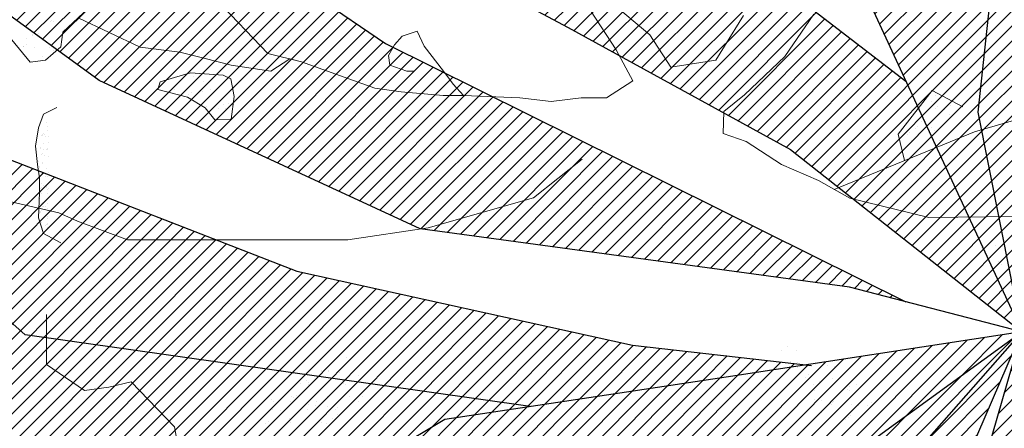
# Model space of a CAD drawing. Units: inches. Extents: x 1986 to 21484, y -1816 to 2016.
# Tile 20 of 85: x 2157.68 to 2172.01, y 1882.44 to 1888.38. Entities that reach past the tile are written whole.
import ezdxf

# ---------------------------------------------------------------- set-up
doc = ezdxf.new("R2010")
doc.units = ezdxf.units.IN
doc.layers.add('L-PLNT', color=84, linetype='Continuous', lineweight=13)
doc.layers.add('vfolhas', color=114, linetype='Continuous', lineweight=5)
for name, color, linetype in [('vfolha', 72, 'Continuous'), ('vfolha2', 110, 'Continuous'), ('vfolhas2', 102, 'Continuous')]:
    doc.layers.add(name, color=color, linetype=linetype)
pattern_1 = [(45, (-2446.5133113, 50.986076), (-0.004419417382, 0.004419417382), [])]

# ---------------------------------------------------------------- blocks, each defined once
blk = doc.blocks.new('arbusto_PB_verde_grande')
at = {"layer": 'vfolha2'}
h = blk.add_hatch(dxfattribs=at)
h.set_pattern_fill('ANSI31', color=256, scale=0.05, style=0)
h.set_pattern_definition(pattern_1)
h.paths.add_polyline_path([(0.02944, 0.35651), (0.00028, 0.09048), (0.02625, -0.03934), (0.047, 0.06233), (0.06189, 0.09731), (0.09372, 0.26573), (0.09955, 0.43473), (0.08789, 0.61313), (0.0645, 0.72266), (0.04988, 0.6851), (0.0236, 0.51294)])
h.paths.add_polyline_path([(0.30106, 0.43789), (0.14225, 0.24871), (0.26685, 0.30022)])
h.paths.add_polyline_path([(0.37995, 0.22817), (0.23697, 0.15193), (0.18428, 0.09364), (0.11122, 0.04358), (0.02625, -0.03934), (0.28061, 0.04667), (0.36829, 0.07798), (0.46756, 0.11239), (0.61068, 0.19376), (0.71585, 0.27823), (0.55813, 0.25948)])
h.paths.add_polyline_path([(0.56101, -0.29441), (0.72752, -0.32573), (0.59024, -0.2412), (0.42962, -0.15982), (0.02625, -0.03934), (0.14922, -0.14107), (0.18838, -0.16604), (0.41501, -0.24435)])
h.paths.add_polyline_path([(-0.27429, -0.44776), (-0.30352, -0.72628), (-0.23923, -0.64175), (-0.15457, -0.45716), (0.02625, -0.03934), (-0.16328, -0.25376)])
h.paths.add_polyline_path([(-0.51963, -0.24744), (-0.67736, -0.32573), (-0.59558, -0.35072), (-0.40574, -0.32882), (-0.21007, -0.20995), (0.02625, -0.03934), (-0.14874, -0.06595), (-0.31518, -0.09101), (-0.41452, -0.15048)])
h.paths.add_polyline_path([(-0.52546, 0.25007), (-0.70947, 0.24698), (-0.51963, 0.1093), (-0.32979, 0.02167), (-0.07567, -0.0128), (-0.04234, -0.02148), (-0.35024, 0.1312)])
at = {"layer": 'vfolhas'}
h = blk.add_hatch(dxfattribs=at)
h.set_pattern_fill('ANSI31', color=256, scale=0.05, style=0)
h.set_pattern_definition(pattern_1)
h.paths.add_polyline_path([(-0.07279, 0.50669), (-0.18085, 0.65063), (-0.2334, 0.67253), (-0.20712, 0.53176), (-0.10785, 0.25007), (0.02625, -0.03934), (0.00028, 0.09048), (0.00816, 0.16241), (-0.04939, 0.29079)])
h.paths.add_polyline_path([(0.09902, 0.41929), (0.09372, 0.26573), (0.07906, 0.18814), (0.15506, 0.36901), (0.26606, 0.5505), (0.28356, 0.63504), (0.2485, 0.68819), (0.25145, 0.63504), (0.20178, 0.54426)])
h.paths.add_polyline_path([(0.12295, 0.24073), (0.047, 0.06233), (0.02625, -0.03934), (0.11122, 0.04358), (0.18428, 0.09364), (0.27478, 0.19376), (0.3215, 0.25323), (0.44129, 0.38467), (0.47634, 0.57866), (0.41789, 0.45347), (0.28939, 0.30954)])
h.paths.add_polyline_path([(0.58145, -0.03779), (0.70707, 0.01536), (0.78591, 0.04667), (0.74796, 0.06549), (0.62818, 0.08423), (0.52595, 0.09048), (0.39745, 0.04358), (0.02625, -0.03934), (0.25728, -0.03154), (0.43834, -0.0347)])
h.paths.add_polyline_path([(0.52022, -0.03647), (0.43834, -0.0347), (0.25728, -0.03154), (0.02625, -0.03934), (0.17964, -0.08515), (0.53768, -0.13167), (0.69541, -0.15357), (0.78591, -0.07852), (0.70413, -0.10042)])
h.paths.add_polyline_path([(0.27189, -0.21929), (0.14922, -0.14107), (0.02625, -0.03934), (0.15794, -0.31007), (0.29522, -0.42585), (0.41789, -0.49157), (0.56396, -0.56669), (0.5114, -0.48532), (0.39456, -0.34139)])
h.paths.add_polyline_path([(-0.05818, -0.47591), (-0.02312, -0.61984), (0.047, -0.80134), (0.08494, -0.59794), (0.07911, -0.4071), (0.03527, -0.25376), (0.02625, -0.03934), (-0.03773, -0.26001)])
h.paths.add_polyline_path([(-0.24218, 0.14054), (-0.11073, 0.06858), (0.02625, -0.03934), (-0.04235, 0.10871), (-0.21007, 0.23757), (-0.36485, 0.33145), (-0.47874, 0.40341), (-0.54303, 0.46288), (-0.49041, 0.33145), (-0.39408, 0.22192)])
h = blk.add_hatch(dxfattribs=at)
h.set_pattern_fill('ANSI31', color=256, scale=0.05, style=0)
h.set_pattern_definition(pattern_1)
h.paths.add_polyline_path([(-0.57219, 0.06233), (-0.7153, 0.10298), (-0.67736, 0.08107), (-0.62769, 0.01536), (-0.56347, -0.04095), (-0.26461, -0.0834), (-0.14874, -0.06595), (-0.10151, -0.05877), (-0.20418, -0.0472), (-0.40279, -0.00339)])
h.paths.add_polyline_path([(-0.56347, -0.04095), (-0.58279, -0.02401), (-0.72992, -0.09726), (-0.4334, -0.1679), (-0.41452, -0.15048), (-0.31518, -0.09101), (-0.26461, -0.0834)])
h.paths.add_polyline_path([(-0.2769, -0.47267), (-0.27429, -0.44776), (-0.16328, -0.25376), (0.02625, -0.03934), (-0.21007, -0.20995), (-0.2672, -0.24466), (-0.36485, -0.35697), (-0.42907, -0.46341), (-0.47586, -0.60425), (-0.37946, -0.57603)])
at = {"layer": 'vfolha'}
for q in [(-0.14874, -0.06595), (-0.03773, -0.26001)]:
    blk.add_line((0.02625, -0.03934), q, dxfattribs=at)
at = {"layer": 'vfolha2'}
for p, q in [((0.00028, 0.09048), (0.02944, 0.35651)), ((-0.51963, 0.1093), (-0.70947, 0.24698)), ((-0.52546, 0.25007), (-0.35024, 0.1312)), ((-0.35024, 0.1312), (-0.04234, -0.02148)), ((-0.32979, 0.02167), (-0.51963, 0.1093)), ((0.02625, -0.03934), (0.00028, 0.09048)), ((-0.07567, -0.0128), (-0.32979, 0.02167)), ((-0.21007, -0.20995), (0.02625, -0.03934)), ((0.02625, -0.03934), (-0.16328, -0.25376)), ((-0.15457, -0.45716), (0.02625, -0.03934)), ((-0.14874, -0.06595), (-0.31518, -0.09101)), ((-0.31518, -0.09101), (-0.41452, -0.15048))]:
    blk.add_line(p, q, dxfattribs=at)
at = {"layer": 'vfolhas2'}
for p, q in [((-0.10785, 0.25007), (0.02625, -0.03934)), ((-0.04235, 0.10871), (-0.21007, 0.23757)), ((-0.39408, 0.22192), (-0.24218, 0.14054)), ((-0.24218, 0.14054), (-0.11073, 0.06858)), ((-0.11073, 0.06858), (0.02625, -0.03934)), ((-0.57219, 0.06233), (-0.40279, -0.00339)), ((-0.56347, -0.04095), (-0.62769, 0.01536)), ((-0.40279, -0.00339), (-0.20418, -0.0472)), ((0.02625, -0.03934), (-0.07567, -0.0128)), ((-0.26461, -0.0834), (-0.56347, -0.04095)), ((-0.20418, -0.0472), (-0.09832, -0.05913))]:
    blk.add_line(p, q, dxfattribs=at)
blk = doc.blocks.new('PLANT-SHRUB')
for p, q in [((2158.755, 1888.613), (2158.308, 1888.194)), ((2161.292, 1887.888), (2160.54, 1888.674)), ((2166.278, 1888.644), (2166.852, 1888.156)), ((2166.362, 1887.939), (2165.989, 1888.51)), ((2167.94, 1887.993), (2168.214, 1888.439)), ((2169.239, 1888.457), (2168.816, 1887.842)), ((2158.122, 1888.357), (2158.122, 1888.357)), ((2158.147, 1888.364), (2158.147, 1888.364)), ((2158.169, 1888.344), (2158.169, 1888.344)), ((2159.433, 1887.976), (2158.532, 1888.403)), ((2157.865, 1888.151), (2157.865, 1888.151)), ((2157.868, 1888.157), (2157.868, 1888.157)), ((2157.948, 1888.182), (2157.948, 1888.182)), ((2158.308, 1888.194), (2158.28, 1887.984)), ((2163.248, 1888.139), (2163.136, 1888.01)), ((2163.464, 1888.209), (2163.248, 1888.139)), ((2163.567, 1887.993), (2163.464, 1888.209)), ((2166.852, 1888.156), (2167.16, 1887.685)), ((2157.833, 1887.761), (2157.567, 1888.082)), ((2157.733, 1887.988), (2157.733, 1887.988)), ((2157.738, 1887.989), (2157.738, 1887.989)), ((2157.775, 1888.023), (2157.775, 1888.023)), ((2157.781, 1888.097), (2157.781, 1888.097)), ((2158.28, 1887.984), (2158.057, 1887.789)), ((2159.433, 1887.976), (2159.433, 1887.976)), ((2160.01, 1887.906), (2159.433, 1887.976)), ((2163.136, 1888.01), (2163.049, 1887.855)), ((2163.766, 1887.734), (2163.567, 1887.993)), ((2167.812, 1887.788), (2167.94, 1887.993)), ((2157.895, 1887.966), (2157.895, 1887.966)), ((2158.007, 1887.844), (2158.007, 1887.844)), ((2158.109, 1887.972), (2158.109, 1887.972)), ((2158.167, 1887.931), (2158.167, 1887.931)), ((2160.359, 1887.819), (2160.01, 1887.906)), ((2161.781, 1887.766), (2161.292, 1887.888)), ((2163.049, 1887.855), (2163.067, 1887.717)), ((2166.362, 1887.939), (2166.362, 1887.939)), ((2166.606, 1887.486), (2166.362, 1887.939)), ((2168.816, 1887.842), (2168.231, 1887.286)), ((2158.057, 1887.789), (2157.833, 1887.761)), ((2157.856, 1887.772), (2157.856, 1887.772)), ((2160.761, 1887.714), (2160.359, 1887.819)), ((2161.338, 1887.627), (2160.761, 1887.714)), ((2161.611, 1887.808), (2161.338, 1887.627)), ((2161.781, 1887.766), (2161.611, 1887.808)), ((2162.848, 1887.381), (2161.781, 1887.766)), ((2163.067, 1887.717), (2163.317, 1887.63)), ((2163.913, 1887.544), (2163.766, 1887.734)), ((2167.16, 1887.685), (2167.812, 1887.788)), ((2160.165, 1887.605), (2159.932, 1887.536)), ((2160.64, 1887.57), (2160.165, 1887.605)), ((2160.753, 1887.518), (2160.64, 1887.57)), ((2163.317, 1887.63), (2163.421, 1887.63)), ((2159.725, 1887.475), (2159.69, 1887.363)), ((2159.932, 1887.536), (2159.725, 1887.475)), ((2160.21, 1887.544), (2160.21, 1887.544)), ((2160.351, 1887.48), (2160.351, 1887.48)), ((2160.804, 1887.259), (2160.753, 1887.518)), ((2163.991, 1887.441), (2163.913, 1887.544)), ((2164.141, 1887.277), (2163.991, 1887.441)), ((2166.606, 1887.486), (2166.221, 1887.242)), ((2159.69, 1887.363), (2160.122, 1887.251)), ((2159.94, 1887.356), (2159.94, 1887.356)), ((2160.141, 1887.287), (2160.141, 1887.287)), ((2160.177, 1887.321), (2160.177, 1887.321)), ((2160.335, 1887.339), (2160.335, 1887.339)), ((2160.451, 1887.359), (2160.451, 1887.359)), ((2160.761, 1886.932), (2160.804, 1887.259)), ((2163.232, 1887.329), (2162.848, 1887.381)), ((2163.844, 1887.277), (2163.232, 1887.329)), ((2164.141, 1887.277), (2163.844, 1887.277)), ((2164.963, 1887.242), (2164.141, 1887.277)), ((2168.231, 1887.286), (2167.929, 1887.04)), ((2170.469, 1886.715), (2170.965, 1887.348)), ((2170.965, 1887.348), (2171.41, 1887.108)), ((2171.011, 1887.275), (2171.011, 1887.275)), ((2160.122, 1887.251), (2160.381, 1887.095)), ((2160.401, 1887.119), (2160.401, 1887.119)), ((2160.654, 1887.145), (2160.654, 1887.145)), ((2160.721, 1887.152), (2160.721, 1887.152)), ((2160.778, 1887.146), (2160.778, 1887.146)), ((2165.417, 1887.189), (2164.963, 1887.242)), ((2165.854, 1887.242), (2165.417, 1887.189)), ((2165.854, 1887.242), (2165.854, 1887.242)), ((2166.221, 1887.242), (2165.854, 1887.242)), ((2170.958, 1887.191), (2170.958, 1887.191)), ((2171.045, 1887.117), (2171.045, 1887.117)), ((2171.234, 1887.125), (2171.234, 1887.125)), ((2171.581, 1886.748), (2172.884, 1887.124)), ((2157.955, 1886.806), (2158.026, 1887.003)), ((2158.026, 1887.003), (2158.223, 1887.101)), ((2158.026, 1887.003), (2158.026, 1887.003)), ((2160.381, 1887.095), (2160.519, 1886.923)), ((2160.57, 1887.091), (2160.57, 1887.091)), ((2160.672, 1887.084), (2160.672, 1887.084)), ((2160.741, 1887.112), (2160.741, 1887.112)), ((2160.776, 1887.07), (2160.776, 1887.07)), ((2167.929, 1887.04), (2167.921, 1886.722)), ((2171.008, 1887.084), (2171.008, 1887.084)), ((2171.149, 1887.072), (2171.149, 1887.072)), ((2171.216, 1886.993), (2171.216, 1886.993)), ((2158.072, 1886.879), (2158.072, 1886.879)), ((2158.089, 1886.83), (2158.089, 1886.83)), ((2160.519, 1886.923), (2160.761, 1886.932)), ((2160.542, 1886.93), (2160.542, 1886.93)), ((2170.81, 1886.901), (2170.81, 1886.901)), ((2157.913, 1886.538), (2157.955, 1886.806)), ((2158.003, 1886.695), (2158.003, 1886.695)), ((2158.011, 1886.692), (2158.011, 1886.692)), ((2158.017, 1886.708), (2158.017, 1886.708)), ((2158.025, 1886.722), (2158.025, 1886.722)), ((2158.043, 1886.712), (2158.043, 1886.712)), ((2158.055, 1886.685), (2158.055, 1886.685)), ((2158.082, 1886.768), (2158.082, 1886.768)), ((2167.921, 1886.722), (2168.255, 1886.608)), ((2169.538, 1885.91), (2171.581, 1886.748)), ((2170.56, 1886.329), (2170.469, 1886.715)), ((2170.599, 1886.708), (2170.599, 1886.708)), ((2170.636, 1886.742), (2170.636, 1886.742)), ((2170.723, 1886.795), (2170.723, 1886.795)), ((2170.753, 1886.819), (2170.753, 1886.819)), ((2170.827, 1886.781), (2170.827, 1886.781)), ((2170.946, 1886.806), (2170.946, 1886.806)), ((2170.99, 1886.76), (2170.99, 1886.76)), ((2158.02, 1886.578), (2158.02, 1886.578)), ((2158.094, 1886.68), (2158.094, 1886.68)), ((2158.096, 1886.597), (2158.096, 1886.597)), ((2168.255, 1886.608), (2168.771, 1886.274)), ((2170.664, 1886.627), (2170.664, 1886.627)), ((2170.988, 1886.571), (2170.988, 1886.571)), ((2171.072, 1886.625), (2171.072, 1886.625)), ((2157.941, 1886.271), (2157.913, 1886.538)), ((2157.982, 1886.524), (2157.982, 1886.524)), ((2157.986, 1886.5), (2157.986, 1886.5)), ((2158, 1886.42), (2158, 1886.42)), ((2158.015, 1886.434), (2158.015, 1886.434)), ((2158.025, 1886.495), (2158.025, 1886.495)), ((2158.035, 1886.409), (2158.035, 1886.409)), ((2158.075, 1886.489), (2158.075, 1886.489)), ((2158.086, 1886.487), (2158.086, 1886.487)), ((2158.089, 1886.501), (2158.089, 1886.501)), ((2157.941, 1886.271), (2157.941, 1886.271)), ((2157.969, 1886.074), (2157.941, 1886.271)), ((2157.956, 1886.31), (2157.956, 1886.31)), ((2158.01, 1886.289), (2158.01, 1886.289)), ((2158.017, 1886.302), (2158.017, 1886.302)), ((2158.095, 1886.389), (2158.095, 1886.389)), ((2165.16, 1885.786), (2165.869, 1886.351)), ((2168.771, 1886.274), (2169.31, 1886.039)), ((2157.966, 1886.244), (2157.966, 1886.244)), ((2157.975, 1886.222), (2157.975, 1886.222)), ((2157.993, 1886.142), (2157.993, 1886.142)), ((2158.006, 1886.145), (2158.006, 1886.145)), ((2158.007, 1886.154), (2158.007, 1886.154)), ((2158.063, 1886.129), (2158.063, 1886.129)), ((2158.072, 1886.214), (2158.072, 1886.214)), ((2158.094, 1886.149), (2158.094, 1886.149)), ((2157.969, 1885.863), (2157.969, 1886.074)), ((2158.001, 1886), (2158.001, 1886)), ((2158.05, 1886.104), (2158.05, 1886.104)), ((2158.089, 1886.099), (2158.089, 1886.099)), ((2169.31, 1886.039), (2169.765, 1885.781)), ((2157.955, 1885.497), (2157.969, 1885.863)), ((2157.981, 1885.919), (2157.981, 1885.919)), ((2157.99, 1885.867), (2157.99, 1885.867)), ((2157.996, 1885.856), (2157.996, 1885.856)), ((2158.002, 1885.941), (2158.002, 1885.941)), ((2158.02, 1885.914), (2158.02, 1885.914)), ((2158.02, 1885.914), (2158.02, 1885.914)), ((2158.034, 1885.961), (2158.034, 1885.961)), ((2158.064, 1885.935), (2158.064, 1885.935)), ((2158.078, 1885.948), (2158.078, 1885.948)), ((2158.081, 1885.906), (2158.081, 1885.906)), ((2158.087, 1885.846), (2158.087, 1885.846)), ((2158.098, 1885.926), (2158.098, 1885.926)), ((2157.329, 1885.781), (2158.252, 1885.568)), ((2157.973, 1885.774), (2157.973, 1885.774)), ((2157.991, 1885.712), (2157.991, 1885.712)), ((2158.011, 1885.721), (2158.011, 1885.721)), ((2158.086, 1885.709), (2158.086, 1885.709)), ((2158.093, 1885.782), (2158.093, 1885.782)), ((2158.093, 1885.782), (2158.093, 1885.782)), ((2163.626, 1885.349), (2165.16, 1885.786)), ((2169.765, 1885.781), (2170.913, 1885.503)), ((2157.983, 1885.588), (2157.983, 1885.588)), ((2157.987, 1885.567), (2157.987, 1885.567)), ((2157.996, 1885.601), (2157.996, 1885.601)), ((2158.007, 1885.659), (2158.007, 1885.659)), ((2158.027, 1885.658), (2158.027, 1885.658)), ((2158.062, 1885.66), (2158.062, 1885.66)), ((2158.088, 1885.638), (2158.088, 1885.638)), ((2158.252, 1885.568), (2158.52, 1885.446)), ((2157.955, 1885.497), (2157.955, 1885.497)), ((2158.026, 1885.271), (2157.955, 1885.497)), ((2157.999, 1885.432), (2157.999, 1885.432)), ((2158.044, 1885.523), (2158.044, 1885.523)), ((2158.081, 1885.421), (2158.081, 1885.421)), ((2158.083, 1885.518), (2158.083, 1885.518)), ((2158.083, 1885.493), (2158.083, 1885.493)), ((2158.086, 1885.398), (2158.086, 1885.398)), ((2158.52, 1885.446), (2159.249, 1885.179)), ((2158.52, 1885.446), (2158.52, 1885.446)), ((2170.913, 1885.503), (2172.174, 1885.515)), ((2158.279, 1885.131), (2158.026, 1885.271)), ((2158.054, 1885.381), (2158.054, 1885.381)), ((2158.054, 1885.378), (2158.054, 1885.378)), ((2158.068, 1885.394), (2158.068, 1885.394)), ((2158.079, 1885.349), (2158.079, 1885.349)), ((2162.459, 1885.179), (2163.626, 1885.349)), ((2159.249, 1885.179), (2160.222, 1885.179)), ((2160.222, 1885.179), (2161.17, 1885.179)), ((2161.17, 1885.179), (2162.459, 1885.179)), ((2171.676, 1885.061), (2171.676, 1885.061)), ((2171.748, 1885.068), (2171.748, 1885.068)), ((2171.784, 1885.103), (2171.784, 1885.103)), ((2171.888, 1885.089), (2171.888, 1885.089)), ((2171.984, 1885.074), (2171.984, 1885.074)), ((2171.773, 1884.881), (2171.773, 1884.881)), ((2171.81, 1884.915), (2171.81, 1884.915)), ((2171.934, 1884.863), (2171.934, 1884.863)), ((2171.975, 1884.814), (2171.975, 1884.814)), ((2158.073, 1884.091), (2158.073, 1883.363)), ((2168.775, 1883.571), (2168.775, 1883.571)), ((2168.859, 1883.625), (2168.859, 1883.625)), ((2168.989, 1883.571), (2168.989, 1883.571)), ((2162.29, 1883.45), (2162.29, 1883.45)), ((2162.439, 1883.465), (2162.439, 1883.465)), ((2168.895, 1883.414), (2168.895, 1883.414)), ((2168.999, 1883.4), (2168.999, 1883.4)), ((2158.073, 1883.363), (2158.626, 1882.986)), ((2158.073, 1883.363), (2158.073, 1883.363)), ((2162.072, 1883.277), (2162.072, 1883.277)), ((2162.079, 1883.257), (2162.079, 1883.257)), ((2162.116, 1883.291), (2162.116, 1883.291)), ((2162.156, 1883.33), (2162.156, 1883.33)), ((2162.169, 1883.278), (2162.169, 1883.278)), ((2162.176, 1883.264), (2162.176, 1883.264)), ((2169.001, 1883.318), (2169.001, 1883.318)), ((2169.162, 1883.379), (2169.162, 1883.379)), ((2169.258, 1883.364), (2169.258, 1883.364)), ((2169.335, 1883.373), (2169.335, 1883.373)), ((2169.433, 1883.343), (2169.433, 1883.343)), ((2169.537, 1883.329), (2169.537, 1883.329)), ((2158.978, 1883.036), (2159.305, 1883.111)), ((2159.305, 1883.111), (2159.933, 1882.458)), ((2159.305, 1883.111), (2159.305, 1883.111)), ((2159.305, 1883.111), (2159.305, 1883.111)), ((2161.852, 1883.137), (2161.852, 1883.137)), ((2162.338, 1883.242), (2162.338, 1883.242)), ((2162.475, 1883.136), (2162.475, 1883.136)), ((2162.61, 1883.207), (2162.61, 1883.207)), ((2169.124, 1883.18), (2169.124, 1883.18)), ((2169.161, 1883.213), (2169.161, 1883.213)), ((2169.32, 1883.123), (2169.32, 1883.123)), ((2169.516, 1883.166), (2169.516, 1883.166)), ((2158.626, 1882.986), (2158.978, 1883.036)), ((2161.768, 1883.083), (2161.768, 1883.083)), ((2161.88, 1883.075), (2161.88, 1883.075)), ((2161.887, 1883.1), (2161.887, 1883.1)), ((2162.39, 1883.082), (2162.39, 1883.082)), ((2162.427, 1883.08), (2162.427, 1883.08)), ((2169.236, 1883.069), (2169.236, 1883.069)), ((2169.246, 1882.979), (2169.246, 1882.979)), ((2169.725, 1883.004), (2169.725, 1883.004)), ((2169.757, 1882.981), (2169.757, 1882.981)), ((2169.762, 1883.038), (2169.762, 1883.038)), ((2169.858, 1883.068), (2169.858, 1883.068)), ((2161.35, 1882.855), (2161.35, 1882.855)), ((2161.372, 1882.831), (2161.372, 1882.831)), ((2161.454, 1882.841), (2161.454, 1882.841)), ((2161.616, 1882.82), (2161.616, 1882.82)), ((2161.633, 1882.9), (2161.633, 1882.9)), ((2161.67, 1882.882), (2161.67, 1882.882)), ((2161.707, 1882.915), (2161.707, 1882.915)), ((2161.994, 1882.83), (2161.994, 1882.83)), ((2162.157, 1882.893), (2162.157, 1882.893)), ((2162.481, 1882.899), (2162.481, 1882.899)), ((2162.617, 1882.828), (2162.617, 1882.828)), ((2162.668, 1882.895), (2162.668, 1882.895)), ((2169.249, 1882.85), (2169.249, 1882.85)), ((2169.353, 1882.836), (2169.353, 1882.836)), ((2169.462, 1882.816), (2169.462, 1882.816)), ((2169.526, 1882.822), (2169.526, 1882.822)), ((2161.363, 1882.712), (2161.363, 1882.712)), ((2161.471, 1882.699), (2161.471, 1882.699)), ((2161.874, 1882.715), (2161.874, 1882.715)), ((2161.888, 1882.784), (2161.888, 1882.784)), ((2161.992, 1882.771), (2161.992, 1882.771)), ((2162.154, 1882.749), (2162.154, 1882.749)), ((2162.271, 1882.706), (2162.271, 1882.706)), ((2162.307, 1882.74), (2162.307, 1882.74)), ((2162.414, 1882.695), (2162.414, 1882.695)), ((2162.426, 1882.713), (2162.426, 1882.713)), ((2169.504, 1882.781), (2169.504, 1882.781)), ((2169.516, 1882.815), (2169.516, 1882.815)), ((2169.787, 1882.779), (2169.787, 1882.779)), ((2169.891, 1882.765), (2169.891, 1882.765)), ((2170.027, 1882.775), (2170.027, 1882.775)), ((2170.053, 1882.744), (2170.053, 1882.744)), ((2170.084, 1882.815), (2170.084, 1882.815)), ((2161.297, 1882.54), (2161.297, 1882.54)), ((2161.607, 1882.583), (2161.607, 1882.583)), ((2161.691, 1882.636), (2161.691, 1882.636)), ((2162.229, 1882.581), (2162.229, 1882.581)), ((2162.313, 1882.635), (2162.313, 1882.635)), ((2169.352, 1882.663), (2169.352, 1882.663)), ((2169.697, 1882.568), (2169.697, 1882.568)), ((2169.744, 1882.596), (2169.744, 1882.596)), ((2169.781, 1882.622), (2169.781, 1882.622)), ((2159.933, 1882.458), (2159.983, 1882.182)), ((2161.26, 1882.506), (2161.26, 1882.506)), ((2161.621, 1882.514), (2161.621, 1882.514)), ((2162.072, 1882.524), (2162.072, 1882.524)), ((2162.144, 1882.508), (2162.144, 1882.508))]:
    blk.add_line(p, q)

msp = doc.modelspace()

# ---------------------------------------------------------------- block references
at = {"layer": 'L-PLNT'}
msp.add_blockref('PLANT-SHRUB', (0, 0), dxfattribs=at)
at = {"layer": 'L-PLNT', "xscale": 24.60366729364114, "yscale": 24.60366729364114, "zscale": 24.60366729364114}
msp.add_blockref('arbusto_PB_verde_grande', (2171.623, 1884.805), dxfattribs=at)

doc.saveas('drawing.dxf')
